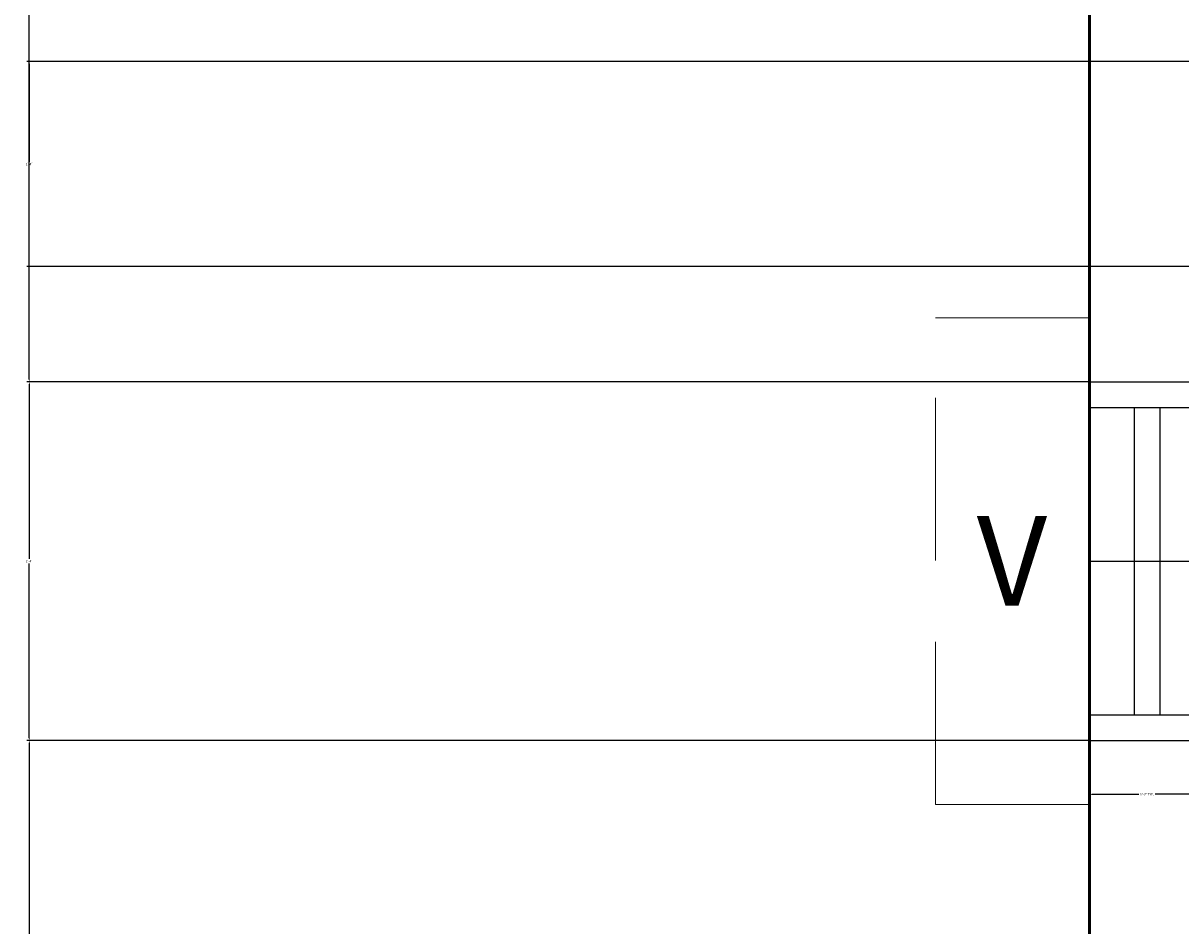
# Model space of a CAD drawing. Units: inches. Extents: x 37 to 824, y -700 to 234.
# Tile 42 of 77: x 78 to 168, y 8 to 78. Entities that reach past the tile are written whole.
import ezdxf

# ---------------------------------------------------------------- set-up
doc = ezdxf.new("R2010")
doc.units = ezdxf.units.IN
doc.header["$MEASUREMENT"] = 0
doc.linetypes.add('DASHED', pattern=[19.05, 12.7, -6.35])
for name, color, linetype, lineweight in [('A-ANNO-DIMS', 2, 'Continuous', 18), ('A-ANNO-TEXT', 7, 'Continuous', 18), ('A-GLAZ', 4, 'Continuous', 25), ('A-ROOF-OVHD', 1, 'DASHED', 18), ('A-WALL', 2, 'Continuous', 50)]:
    doc.layers.add(name, color=color, linetype=linetype, lineweight=lineweight)
doc.styles.get("Standard").update_dxf_attribs({"font": 'arial.ttf'})
doc.dimstyles.get("Standard").update_dxf_attribs({"dimtxt": 0.18, "dimasz": 0.18, "dimexe": 0.18, "dimexo": 0.0625, "dimgap": 0.09, "dimtad": 0, "dimtih": 1, "dimtoh": 1, "dimdec": 1, "dimzin": 0, "dimdsep": 46, "dimlunit": 4, "dimtxsty": 'Standard', "dimcen": 0.09, "dimadec": 0, "dimazin": 0, "dimtfac": 1, "dimtdec": 1, "dimtofl": 0, "dimtmove": 0, "dimatfit": 3, "dimfxl": 1, "dimtolj": 1, "dimtzin": 0, "dimarcsym": 0})

# ---------------------------------------------------------------- blocks, each defined once
blk = doc.blocks.new('VENT-600')
for p, q in [((0, 28), (9, 28)), ((0, 26), (9, 26)), ((3.5, 26), (3.5, 2)), ((5.5, 26), (5.5, 2)), ((0, 14), (9, 14)), ((0, 2), (9, 2)), ((0, 0), (9, 0))]:
    blk.add_line(p, q)
blk = doc.blocks.new('*D41')
at = {"layer": 'A-ANNO-DIMS', "color": 0, "lineweight": -2, "ltscale": 0.5, "transparency": 16777216}
for p, q in [((161.077, 22.028), (161.077, 17.71)), ((170.077, 22.028), (170.077, 17.71)), ((161.257, 17.89), (164.939, 17.89)), ((169.897, 17.89), (166.216, 17.89))]:
    blk.add_line(p, q, dxfattribs=at)
at = {"layer": 'A-ANNO-DIMS', "color": 0, "ltscale": 0.5, "transparency": 16777216}
for points in [[(161.257, 17.92), (161.257, 17.86), (161.077, 17.89)], [(169.897, 17.92), (169.897, 17.86), (170.077, 17.89)]]:
    blk.add_solid(points, dxfattribs=at)
at = {"layer": 'Defpoints', "color": 0, "ltscale": 0.5, "transparency": 16777216}
for p in [(161.077, 22.09), (170.077, 22.09), (170.077, 17.89)]:
    blk.add_point(p, dxfattribs=at)
at = {"layer": 'A-ANNO-DIMS', "color": 0, "ltscale": 0.5, "transparency": 16777216, "insert": (165.577, 17.89), "char_height": 0.18, "attachment_point": 5}
blk.add_mtext('\\A1;0\'-9" TYP.', dxfattribs=at)
blk = doc.blocks.new('*D51')
at = {"layer": 'A-ANNO-DIMS', "color": 0, "lineweight": -2, "ltscale": 0.5, "transparency": 16777216}
for p, q in [((161.015, 113.09), (78.159, 113.09)), ((78.339, 112.91), (78.339, 81.772)), ((78.339, 50.27), (78.339, 81.408)), ((161.015, 50.09), (78.159, 50.09))]:
    blk.add_line(p, q, dxfattribs=at)
at = {"layer": 'A-ANNO-DIMS', "color": 0, "ltscale": 0.5, "transparency": 16777216}
for points in [[(78.309, 112.91), (78.369, 112.91), (78.339, 113.09)], [(78.309, 50.27), (78.369, 50.27), (78.339, 50.09)]]:
    blk.add_solid(points, dxfattribs=at)
at = {"layer": 'Defpoints', "color": 0, "ltscale": 0.5, "transparency": 16777216}
for p in [(161.077, 113.09), (78.339, 50.09), (161.077, 50.09)]:
    blk.add_point(p, dxfattribs=at)
at = {"layer": 'A-ANNO-DIMS', "color": 0, "ltscale": 0.5, "transparency": 16777216, "insert": (78.339, 81.59), "char_height": 0.18, "attachment_point": 5}
blk.add_mtext('\\A1;5\'-3"', dxfattribs=at)
blk = doc.blocks.new('*D52')
at = {"layer": 'A-ANNO-DIMS', "color": 0, "lineweight": -2, "ltscale": 0.5, "transparency": 16777216}
for p, q in [((161.015, 50.09), (78.159, 50.09)), ((78.339, 49.91), (78.339, 36.271)), ((78.339, 22.27), (78.339, 35.91)), ((161.015, 22.09), (78.159, 22.09))]:
    blk.add_line(p, q, dxfattribs=at)
at = {"layer": 'A-ANNO-DIMS', "color": 0, "ltscale": 0.5, "transparency": 16777216}
for points in [[(78.309, 49.91), (78.369, 49.91), (78.339, 50.09)], [(78.309, 22.27), (78.369, 22.27), (78.339, 22.09)]]:
    blk.add_solid(points, dxfattribs=at)
at = {"layer": 'Defpoints', "color": 0, "ltscale": 0.5, "transparency": 16777216}
for p in [(161.077, 50.09), (78.339, 22.09), (161.077, 22.09)]:
    blk.add_point(p, dxfattribs=at)
at = {"layer": 'A-ANNO-DIMS', "color": 0, "ltscale": 0.5, "transparency": 16777216, "insert": (78.339, 36.09), "char_height": 0.18, "attachment_point": 5}
blk.add_mtext('\\A1;2\'-4"', dxfattribs=at)
blk = doc.blocks.new('*D53')
at = {"layer": 'A-ANNO-DIMS', "color": 0, "lineweight": -2, "ltscale": 0.5, "transparency": 16777216}
for p, q in [((161.015, 22.09), (78.159, 22.09)), ((78.339, 21.91), (78.339, -3.476)), ((78.339, -29.23), (78.339, -3.843)), ((161.015, -29.41), (78.159, -29.41))]:
    blk.add_line(p, q, dxfattribs=at)
at = {"layer": 'A-ANNO-DIMS', "color": 0, "ltscale": 0.5, "transparency": 16777216}
for points in [[(78.309, 21.91), (78.369, 21.91), (78.339, 22.09)], [(78.309, -29.23), (78.369, -29.23), (78.339, -29.41)]]:
    blk.add_solid(points, dxfattribs=at)
at = {"layer": 'Defpoints', "color": 0, "ltscale": 0.5, "transparency": 16777216}
for p in [(161.077, 22.09), (78.339, -29.41), (161.077, -29.41)]:
    blk.add_point(p, dxfattribs=at)
at = {"layer": 'A-ANNO-DIMS', "color": 0, "ltscale": 0.5, "transparency": 16777216, "insert": (78.339, -3.66), "char_height": 0.18, "attachment_point": 5}
blk.add_mtext('\\A1;4\'-3 1/2"', dxfattribs=at)
blk = doc.blocks.new('*D61')
at = {"layer": 'A-ANNO-DIMS', "color": 0, "lineweight": -2, "ltscale": 0.5, "transparency": 16777216}
for p, q in [((419.015, 75.09), (78.159, 75.09)), ((78.339, 74.91), (78.339, 67.271)), ((78.339, 59.27), (78.339, 66.91)), ((419.015, 59.09), (78.159, 59.09))]:
    blk.add_line(p, q, dxfattribs=at)
at = {"layer": 'A-ANNO-DIMS', "color": 0, "ltscale": 0.5, "transparency": 16777216}
for points in [[(78.309, 74.91), (78.369, 74.91), (78.339, 75.09)], [(78.309, 59.27), (78.369, 59.27), (78.339, 59.09)]]:
    blk.add_solid(points, dxfattribs=at)
at = {"layer": 'Defpoints', "color": 0, "ltscale": 0.5, "transparency": 16777216}
for p in [(419.077, 75.09), (78.339, 59.09), (419.077, 59.09)]:
    blk.add_point(p, dxfattribs=at)
at = {"layer": 'A-ANNO-DIMS', "color": 0, "ltscale": 0.5, "transparency": 16777216, "insert": (78.339, 67.09), "char_height": 0.18, "attachment_point": 5}
blk.add_mtext('\\A1;1\'-4"', dxfattribs=at)

msp = doc.modelspace()

# ---------------------------------------------------------------- linework, layer by layer
at = {"layer": 'A-ROOF-OVHD'}
for p, q in [((161.077, 55.09), (149.077, 55.09)), ((149.077, 17.09), (149.077, 55.09)), ((161.077, 50.09), (161.077, 55.09)), ((161.077, 22.09), (161.077, 17.09)), ((161.077, 17.09), (149.077, 17.09))]:
    msp.add_line(p, q, dxfattribs=at)
at = {"layer": 'A-WALL'}
for q in [(161.077, 191.09), (161.077, -365.91)]:
    msp.add_line((161.077, 75.09), q, dxfattribs=at)

# ---------------------------------------------------------------- block references
at = {"layer": 'A-GLAZ'}
msp.add_blockref('VENT-600', (161.077, 22.09), dxfattribs=at)

# ---------------------------------------------------------------- texts
at = {"layer": 'A-ANNO-TEXT'}
msp.add_text('V', height=7, dxfattribs=at).set_placement((152.282, 32.618))

# ---------------------------------------------------------------- dimensions: what is measured, and where the dimension line sits
at = {"layer": 'A-ANNO-DIMS', "ltscale": 0.5}
for base, p1, p2, picture, middle in [((78.339, 50.09), (161.077, 113.09), (161.077, 50.09), '*D51', (78.339, 81.59)), ((78.339, 59.09), (419.077, 75.09), (419.077, 59.09), '*D61', (78.339, 67.09)), ((78.339, 22.09), (161.077, 50.09), (161.077, 22.09), '*D52', (78.339, 36.09)), ((78.339, -29.41), (161.077, 22.09), (161.077, -29.41), '*D53', (78.339, -3.66))]:
    dim = msp.add_linear_dim(base=base, p1=p1, p2=p2, angle=90, dimstyle='Standard', override={"dimdec": 1, "dimlfac": 1, "dimrnd": 0, "dimzin": 1, "dimdsep": 46, "dimlunit": 4, "dimfrac": 2}, dxfattribs=at)
    dim.commit()
    dim.dimension.update_dxf_attribs({"geometry": picture, "text_midpoint": middle})
dim = msp.add_linear_dim(base=(170.077, 17.89), p1=(161.077, 22.09), p2=(170.077, 22.09), text='<> TYP.', dimstyle='Standard', override={"dimdec": 1, "dimlfac": 1, "dimrnd": 0, "dimzin": 1, "dimdsep": 46, "dimlunit": 4, "dimfrac": 2}, dxfattribs=at)
dim.commit()
dim.dimension.update_dxf_attribs({"geometry": '*D41', "text_midpoint": (165.577, 17.89)})

doc.saveas('drawing.dxf')
